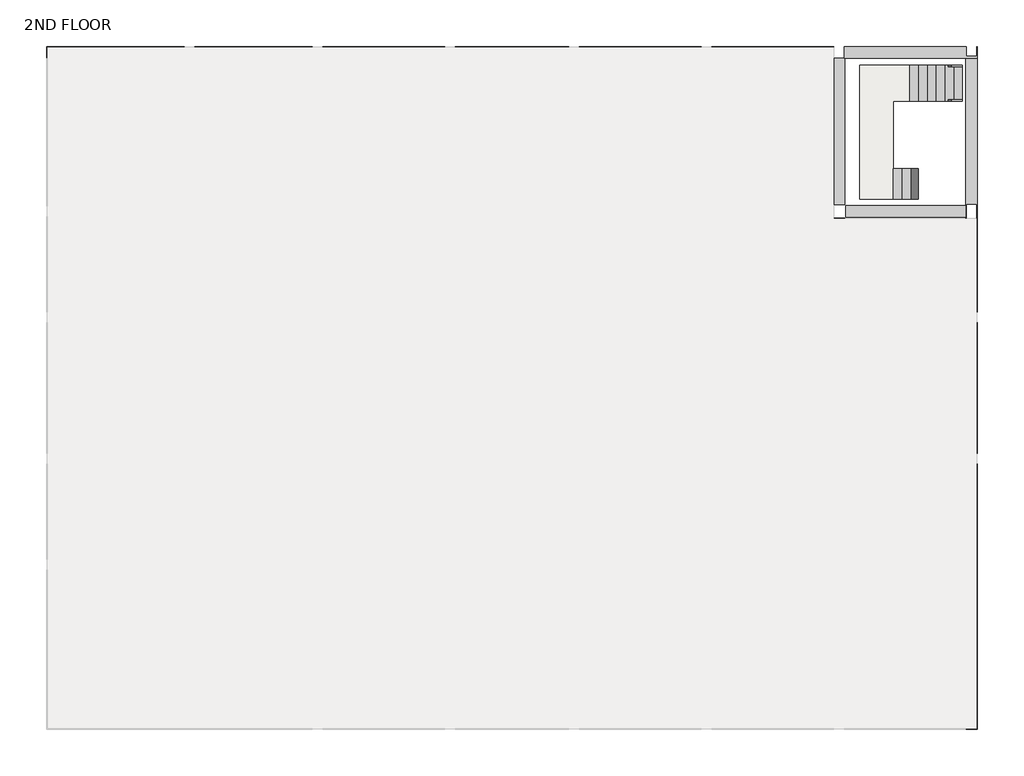
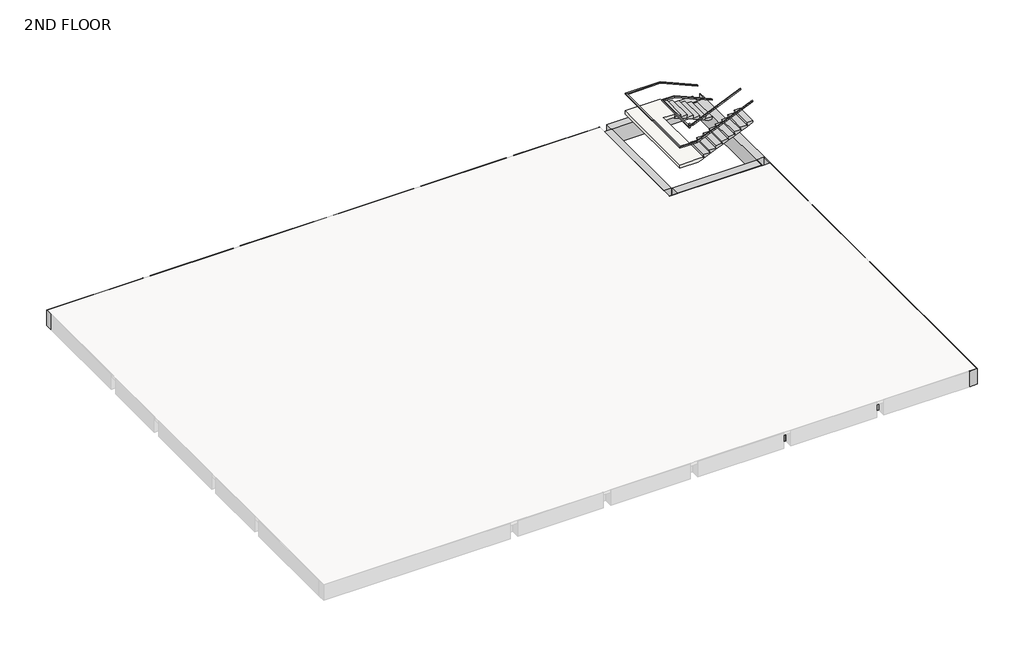
# One storey, part 2 of 2: 5 beams, 2 railings, 2 stair flights, 1 slab.
"""IFC4 building model written with IfcOpenShell, lengths in millimetres."""

from ifc_helpers import new_model, si_unit, frame, origin, place, context, project, spatial, polyline, outline, extrude, faceted_brep, element, save

model = new_model("IFC4")

# Units and contexts
model_context = context("Model", 3, world=origin())
ifc_project = project(units=[si_unit("LENGTHUNIT", "METRE", prefix="MILLI")], contexts=[model_context])

# Site, building, storey
site = spatial("IfcSite", under=ifc_project)
building = spatial("IfcBuilding", under=site)
storey = spatial("IfcBuildingStorey", under=building, Name="2ND FLOOR", Elevation=7620.0)

# Beams
placement = place(None, origin())
element("IfcBeam", 1, ObjectType="M_Concrete-Rectangular Beam : 400 x 800mm", at=placement, inside=storey, context=model_context, shape_type="Brep", body=[
    faceted_brep([(6397.6508981, 16716.9690835, 7620.0), (6397.6508981, 17116.9690835, 7620.0), (6375.4508981, 17116.9690835, 7620.0), (6375.4508981, 16789.9690835, 7620.0), (6019.8508981, 16789.9690835, 7620.0), (6019.8508981, 17116.9690835, 7620.0), (1803.4508981, 17116.9690835, 7620.0), (1803.4508981, 16716.9690835, 7620.0), (1825.6508981, 16716.9690835, 7620.0), (5997.6508981, 16716.9690835, 7620.0), (6397.6508981, 16716.9690835, 6820.0), (1803.4508981, 16716.9690835, 6820.0), (1825.6508981, 16716.9690835, 6820.0), (5997.6508981, 16716.9690835, 6820.0), (6397.6508981, 17116.9690835, 6820.0), (1803.4508981, 17116.9690835, 6820.0), (6019.8508981, 17116.9690835, 6820.0), (6019.8508981, 16789.9690835, 6820.0), (6375.4508981, 16789.9690835, 6820.0), (6375.4508981, 17116.9690835, 6820.0)], [[[0, 1, 2, 3, 4, 5, 6, 7, 8, 9]], [[10, 0, 9, 8, 7, 11, 12, 13]], [[14, 10, 13, 12, 11, 15, 16, 17, 18, 19]], [[1, 14, 19, 2]], [[1, 0, 10, 14]], [[18, 3, 2, 19]], [[3, 18, 17, 4]], [[4, 17, 16, 5]], [[5, 16, 15, 6]], [[7, 6, 15, 11]]]),
    faceted_brep([(-25701.5491019, 16716.9690835, 7620.0), (-25701.5491019, 17116.9690835, 7620.0), (-25701.5491019, 17116.9690835, 6820.0), (-25701.5491019, 16716.9690835, 6820.0), (-25323.7491019, 17094.7690835, 6820.0), (-25323.7491019, 16739.1690835, 6820.0), (-25323.7491019, 16739.1690835, 7467.6), (-25323.7491019, 17094.7690835, 7467.6), (-25679.3491019, 16739.1690835, 6820.0), (-25679.3491019, 16739.1690835, 7467.6), (-25679.3491019, 16716.9690835, 7620.0), (-25679.3491019, 16716.9690835, 7467.6), (-25679.3491019, 17094.7690835, 6820.0), (-25679.3491019, 17094.7690835, 7467.6), (-25679.3491019, 17094.7690835, 7620.0), (-20954.9491019, 16716.9690835, 6820.0), (-20954.9491019, 17116.9690835, 6820.0), (-20954.9491019, 17116.9690835, 7620.0), (-20954.9491019, 17094.7690835, 7620.0), (-20954.9491019, 17094.7690835, 7467.6), (-20954.9491019, 16716.9690835, 7467.6), (-25301.5491019, 16716.9690835, 6820.0), (-20977.1491019, 16716.9690835, 6820.0), (-20977.1491019, 16716.9690835, 7467.6), (-25301.5491019, 16716.9690835, 7467.6)], [[[0, 1, 2, 3]], [[4, 5, 6, 7]], [[5, 8, 9, 6]], [[10, 11, 9, 8, 12, 13, 14]], [[15, 16, 17, 18, 19, 20]], [[1, 0, 10, 14, 18, 17]], [[0, 3, 21, 22, 15, 20, 23, 24, 11, 10]], [[3, 2, 16, 15, 22, 21], [5, 4, 12, 8]], [[2, 1, 17, 16]], [[14, 13, 12, 4, 7, 19, 18]], [[19, 7, 6, 9, 11, 24, 23, 20]]]),
    faceted_brep([(-2768.5491019, 17094.7690835, 7467.6), (1447.8508981, 17094.7690835, 7467.6), (1447.8508981, 17094.7690835, 7620.0), (-2768.5491019, 17094.7690835, 7620.0), (-2768.5491019, 17116.9690835, 6820.0), (-2768.5491019, 16716.9690835, 6820.0), (-2768.5491019, 16716.9690835, 7467.6), (-2768.5491019, 17116.9690835, 7620.0), (1447.8508981, 16716.9690835, 6820.0), (1447.8508981, 17116.9690835, 6820.0), (1447.8508981, 17116.9690835, 7620.0), (1447.8508981, 16716.9690835, 7467.6), (-2746.3491019, 16716.9690835, 6820.0), (1425.6508981, 16716.9690835, 6820.0), (1425.6508981, 16716.9690835, 7467.6), (-2746.3491019, 16716.9690835, 7467.6)], [[[0, 1, 2, 3]], [[4, 5, 6, 0, 3, 7]], [[8, 9, 10, 2, 1, 11]], [[10, 7, 3, 2]], [[5, 12, 13, 8, 11, 14, 15, 6]], [[5, 4, 9, 8, 13, 12]], [[4, 7, 10, 9]], [[1, 0, 6, 15, 14, 11]]]),
    faceted_brep([(-16179.7491019, 17116.9690835, 6820.0), (-16179.7491019, 16716.9690835, 6820.0), (-16179.7491019, 16716.9690835, 7467.6), (-16179.7491019, 17094.7690835, 7467.6), (-16179.7491019, 17094.7690835, 7620.0), (-16179.7491019, 17116.9690835, 7620.0), (-11963.3491019, 16716.9690835, 6820.0), (-11963.3491019, 17116.9690835, 6820.0), (-11963.3491019, 17116.9690835, 7620.0), (-11963.3491019, 17094.7690835, 7620.0), (-11963.3491019, 17094.7690835, 7467.6), (-11963.3491019, 16716.9690835, 7467.6), (-16157.5491019, 16716.9690835, 6820.0), (-11985.5491019, 16716.9690835, 6820.0), (-11985.5491019, 16716.9690835, 7467.6), (-16157.5491019, 16716.9690835, 7467.6)], [[[0, 1, 2, 3, 4, 5]], [[6, 7, 8, 9, 10, 11]], [[8, 5, 4, 9]], [[1, 12, 13, 6, 11, 14, 15, 2]], [[1, 0, 7, 6, 13, 12]], [[0, 5, 8, 7]], [[3, 10, 9, 4]], [[10, 3, 2, 15, 14, 11]]]),
    faceted_brep([(-16535.3491019, 16716.9690835, 6820.0), (-16535.3491019, 17116.9690835, 6820.0), (-16535.3491019, 17116.9690835, 7620.0), (-16535.3491019, 17094.7690835, 7620.0), (-16535.3491019, 17094.7690835, 7467.6), (-16535.3491019, 16716.9690835, 7467.6), (-20599.3491019, 17116.9690835, 7620.0), (-20599.3491019, 17094.7690835, 7620.0), (-20599.3491019, 16716.9690835, 6820.0), (-20577.1491019, 16716.9690835, 6820.0), (-16557.5491019, 16716.9690835, 6820.0), (-16557.5491019, 16716.9690835, 7467.6), (-20577.1491019, 16716.9690835, 7467.6), (-20599.3491019, 16716.9690835, 7467.6), (-20599.3491019, 17116.9690835, 6820.0), (-20599.3491019, 17094.7690835, 7467.6)], [[[0, 1, 2, 3, 4, 5]], [[2, 6, 7, 3]], [[8, 9, 10, 0, 5, 11, 12, 13]], [[1, 0, 10, 9, 8, 14]], [[2, 1, 14, 6]], [[14, 8, 13, 15, 7, 6]], [[15, 4, 3, 7]], [[4, 15, 13, 12, 11, 5]]]),
    faceted_brep([(-11607.7491019, 17116.9690835, 6820.0), (-11607.7491019, 16716.9690835, 6820.0), (-11607.7491019, 16716.9690835, 7467.6), (-11607.7491019, 17094.7690835, 7467.6), (-11607.7491019, 17094.7690835, 7620.0), (-11607.7491019, 17116.9690835, 7620.0), (-7696.1491019, 16716.9690835, 6820.0), (-7696.1491019, 17116.9690835, 6820.0), (-7696.1491019, 17116.9690835, 7620.0), (-7696.1491019, 17094.7690835, 7620.0), (-7696.1491019, 17094.7690835, 7467.6), (-7696.1491019, 16716.9690835, 7467.6), (-11585.5491019, 16716.9690835, 6820.0), (-7718.3491019, 16716.9690835, 6820.0), (-7718.3491019, 16716.9690835, 7467.6), (-11585.5491019, 16716.9690835, 7467.6)], [[[0, 1, 2, 3, 4, 5]], [[6, 7, 8, 9, 10, 11]], [[8, 5, 4, 9]], [[1, 12, 13, 6, 11, 14, 15, 2]], [[1, 0, 7, 6, 13, 12]], [[0, 5, 8, 7]], [[3, 10, 9, 4]], [[10, 3, 2, 15, 14, 11]]]),
    faceted_brep([(-7340.5491019, 17116.9690835, 6820.0), (-7340.5491019, 16716.9690835, 6820.0), (-7340.5491019, 16716.9690835, 7467.6), (-7340.5491019, 17094.7690835, 7467.6), (-7340.5491019, 17094.7690835, 7620.0), (-7340.5491019, 17116.9690835, 7620.0), (-3124.1491019, 16716.9690835, 6820.0), (-3124.1491019, 17116.9690835, 6820.0), (-3124.1491019, 17116.9690835, 7620.0), (-3124.1491019, 17094.7690835, 7620.0), (-3124.1491019, 17094.7690835, 7467.6), (-3124.1491019, 16716.9690835, 7467.6), (-7318.3491019, 16716.9690835, 6820.0), (-3146.3491019, 16716.9690835, 6820.0), (-3146.3491019, 16716.9690835, 7467.6), (-7318.3491019, 16716.9690835, 7467.6)], [[[0, 1, 2, 3, 4, 5]], [[6, 7, 8, 9, 10, 11]], [[8, 5, 4, 9]], [[1, 12, 13, 6, 11, 14, 15, 2]], [[1, 0, 7, 6, 13, 12]], [[0, 5, 8, 7]], [[3, 10, 9, 4]], [[10, 3, 2, 15, 14, 11]]]),
])
element("IfcBeam", 2, ObjectType="M_Concrete-Rectangular Beam : 400 x 800mm", at=placement, inside=storey, context=model_context, shape_type="Brep", body=[
    faceted_brep([(5997.6508981, -6447.8309165, 7620.0), (6397.6508981, -6447.8309165, 7620.0), (6397.6508981, 2718.3690835, 7620.0), (6375.4508981, 2718.3690835, 7620.0), (6375.4508981, -6425.6309165, 7620.0), (5997.6508981, -6425.6309165, 7620.0), (5997.6508981, -6447.8309165, 6820.0), (5997.6508981, -6425.6309165, 7467.6), (5997.6508981, -6047.8309165, 7467.6), (5997.6508981, -961.4309165, 7467.6), (5997.6508981, -561.4309165, 7467.6), (5997.6508981, 2696.1690835, 7467.6), (5997.6508981, 2718.3690835, 7467.6), (5997.6508981, 2718.3690835, 6820.0), (5997.6508981, 2696.1690835, 6820.0), (5997.6508981, -561.4309165, 6820.0), (5997.6508981, -961.4309165, 6820.0), (5997.6508981, -6047.8309165, 6820.0), (6397.6508981, -6447.8309165, 6820.0), (6397.6508981, 2718.3690835, 6820.0), (6375.4508981, -6425.6309165, 6820.0), (6375.4508981, -6070.0309165, 6820.0), (6019.8508981, -6070.0309165, 6820.0), (6019.8508981, -6425.6309165, 6820.0), (6375.4508981, -1015.4309165, 6820.0), (6375.4508981, -507.4309165, 6820.0), (6019.8508981, -507.4309165, 6820.0), (6019.8508981, -1015.4309165, 6820.0), (6375.4508981, 2718.3690835, 7467.6), (6375.4508981, -507.4309165, 7467.6), (6375.4508981, -1015.4309165, 7467.6), (6375.4508981, -6070.0309165, 7467.6), (6375.4508981, -6425.6309165, 7467.6), (6019.8508981, -6425.6309165, 7467.6), (6019.8508981, -6070.0309165, 7467.6), (6019.8508981, -1015.4309165, 7467.6), (6019.8508981, -507.4309165, 7467.6)], [[[0, 1, 2, 3, 4, 5]], [[6, 0, 5, 7, 8, 9, 10, 11, 12, 13, 14, 15, 16, 17]], [[18, 6, 17, 16, 15, 14, 13, 19], [20, 21, 22, 23], [24, 25, 26, 27]], [[1, 18, 19, 2]], [[1, 0, 6, 18]], [[3, 28, 29, 25, 24, 30, 31, 21, 20, 32, 4]], [[4, 32, 20, 23, 33, 7, 5]], [[23, 22, 34, 33]], [[22, 21, 31, 34]], [[19, 13, 12, 28, 3, 2]], [[24, 27, 35, 30]], [[27, 26, 36, 35]], [[26, 25, 29, 36]], [[31, 30, 35, 36, 29, 28, 12, 11, 10, 9, 8, 7, 33, 34]]]),
    faceted_brep([(5997.6508981, 16716.9690835, 6820.0), (5997.6508981, 16716.9690835, 7620.0), (6397.6508981, 16716.9690835, 7620.0), (6397.6508981, 16716.9690835, 6820.0), (5997.6508981, 7950.7690835, 6820.0), (6397.6508981, 7950.7690835, 6820.0), (6397.6508981, 7950.7690835, 7620.0), (6375.4508981, 7950.7690835, 7620.0), (6375.4508981, 7950.7690835, 7467.6), (5997.6508981, 7950.7690835, 7467.6), (5997.6508981, 11630.5690835, 7620.0), (5997.6508981, 11230.5690835, 7620.0), (5997.6508981, 11176.5690835, 7620.0), (6019.8508981, 11176.5690835, 7620.0), (6019.8508981, 11684.5690835, 7620.0), (6375.4508981, 11684.5690835, 7620.0), (6375.4508981, 11176.5690835, 7620.0), (5997.6508981, 11630.5690835, 6820.0), (5997.6508981, 11230.5690835, 6820.0), (5997.6508981, 7972.9690835, 6820.0), (5997.6508981, 7972.9690835, 7467.6), (5997.6508981, 11176.5690835, 7467.6), (6375.4508981, 11176.5690835, 6820.0), (6375.4508981, 11684.5690835, 6820.0), (6019.8508981, 11684.5690835, 6820.0), (6019.8508981, 11176.5690835, 6820.0), (6019.8508981, 11176.5690835, 7467.6), (6375.4508981, 11176.5690835, 7467.6)], [[[0, 1, 2, 3]], [[4, 5, 6, 7, 8, 9]], [[2, 1, 10, 11, 12, 13, 14, 15, 16, 7, 6]], [[1, 0, 17, 18, 19, 4, 9, 20, 21, 12, 11, 10]], [[0, 3, 5, 4, 19, 18, 17], [22, 23, 24, 25]], [[3, 2, 6, 5]], [[22, 25, 26, 27]], [[24, 14, 13, 26, 25]], [[14, 24, 23, 15]], [[8, 27, 26, 21, 20, 9]], [[27, 8, 7, 16, 15, 23, 22]], [[21, 26, 13, 12]]]),
    faceted_brep([(6397.6508981, 7595.1690835, 6820.0), (5997.6508981, 7595.1690835, 6820.0), (5997.6508981, 7595.1690835, 7467.6), (6375.4508981, 7595.1690835, 7467.6), (6375.4508981, 7595.1690835, 7620.0), (6397.6508981, 7595.1690835, 7620.0), (5997.6508981, 3073.9690835, 6820.0), (6397.6508981, 3073.9690835, 6820.0), (6397.6508981, 3073.9690835, 7620.0), (6375.4508981, 3073.9690835, 7620.0), (6375.4508981, 3073.9690835, 7467.6), (5997.6508981, 3073.9690835, 7467.6), (5997.6508981, 7572.9690835, 6820.0), (5997.6508981, 3096.1690835, 6820.0), (5997.6508981, 3096.1690835, 7467.6), (5997.6508981, 7572.9690835, 7467.6)], [[[0, 1, 2, 3, 4, 5]], [[6, 7, 8, 9, 10, 11]], [[8, 5, 4, 9]], [[1, 12, 13, 6, 11, 14, 15, 2]], [[1, 0, 7, 6, 13, 12]], [[0, 5, 8, 7]], [[3, 10, 9, 4]], [[10, 3, 2, 15, 14, 11]]]),
])
element("IfcBeam", 3, ObjectType="M_Concrete-Rectangular Beam : 400 x 800mm", at=placement, inside=storey, context=model_context, shape_type="SweptSolid", body=[
    extrude(outline(polyline([(-2746.3491019, -6047.8309165), (-2768.5491019, -6047.8309165), (-2768.5491019, -6019.2309165), (-3124.1491019, -6019.2309165), (-3124.1491019, -6047.8309165), (-3146.3491019, -6047.8309165), (-3146.3491019, -990.0309165), (-2746.3491019, -990.0309165), (-2746.3491019, -6047.8309165)])), frame((0.0, 0.0, 6820.0), z_axis=(0.0, 0.0, 1.0), x_axis=(1.0, 0.0, 0.0)), (0.0, 0.0, 1.0), 647.6),
    extrude(outline(polyline([(-2768.5491019, 16716.9690835), (-2746.3491019, 16716.9690835), (-2746.3491019, 11659.1690835), (-3146.3491019, 11659.1690835), (-3146.3491019, 16716.9690835), (-3124.1491019, 16716.9690835), (-3124.1491019, 16688.3690835), (-2768.5491019, 16688.3690835), (-2768.5491019, 16716.9690835)])), frame((0.0, 0.0, 6820.0), z_axis=(0.0, 0.0, 1.0), x_axis=(1.0, 0.0, 0.0)), (0.0, 0.0, 1.0), 647.6),
    extrude(outline(polyline([(-3146.3491019, 11201.9690835), (-2746.3491019, 11201.9690835), (-2746.3491019, 8001.5690835), (-3146.3491019, 8001.5690835), (-3146.3491019, 11201.9690835)])), frame((0.0, 0.0, 6820.0), z_axis=(0.0, 0.0, 1.0), x_axis=(1.0, 0.0, 0.0)), (0.0, 0.0, 1.0), 647.6),
    extrude(outline(polyline([(-3146.3491019, 7544.3690835), (-2746.3491019, 7544.3690835), (-2746.3491019, 3124.7690835), (-3146.3491019, 3124.7690835), (-3146.3491019, 7544.3690835)])), frame((0.0, 0.0, 6820.0), z_axis=(0.0, 0.0, 1.0), x_axis=(1.0, 0.0, 0.0)), (0.0, 0.0, 1.0), 647.6),
    extrude(outline(polyline([(-2746.3491019, -532.8309165), (-3146.3491019, -532.8309165), (-3146.3491019, 2667.5690835), (-2746.3491019, 2667.5690835), (-2746.3491019, -532.8309165)])), frame((0.0, 0.0, 6820.0), z_axis=(0.0, 0.0, 1.0), x_axis=(1.0, 0.0, 0.0)), (0.0, 0.0, 1.0), 647.6),
])
element("IfcBeam", 4, ObjectType="M_Concrete-Rectangular Beam : 400 x 800mm", at=placement, inside=storey, context=model_context, shape_type="Brep", body=[
    faceted_brep([(1425.6508981, -990.0309165, 6820.0), (1425.6508981, -6047.8309165, 6820.0), (1425.6508981, -6047.8309165, 7467.6), (1425.6508981, -990.0309165, 7467.6), (1825.6508981, -6047.8309165, 6820.0), (1803.4508981, -6047.8309165, 6820.0), (1803.4508981, -6019.2309165, 6820.0), (1447.8508981, -6019.2309165, 6820.0), (1447.8508981, -6047.8309165, 6820.0), (1825.6508981, -990.0309165, 6820.0), (1825.6508981, -990.0309165, 7467.6), (1825.6508981, -6047.8309165, 7467.6), (1447.8508981, -6047.8309165, 7467.6), (1803.4508981, -6047.8309165, 7467.6), (1803.4508981, -6019.2309165, 7467.6), (1447.8508981, -6019.2309165, 7467.6)], [[[0, 1, 2, 3]], [[4, 5, 6, 7, 8, 1, 0, 9]], [[4, 9, 10, 11]], [[1, 8, 12, 2]], [[6, 5, 13, 14]], [[8, 7, 15, 12]], [[7, 6, 14, 15]], [[5, 4, 11, 13]], [[9, 0, 3, 10]], [[3, 2, 12, 15, 14, 13, 11, 10]]]),
    faceted_brep([(1825.6508981, 16716.9690835, 7620.0), (1825.6508981, 16716.9690835, 6820.0), (1803.4508981, 16716.9690835, 6820.0), (1803.4508981, 16716.9690835, 7620.0), (1803.4508981, 16713.7690835, 6820.0), (1803.4508981, 16713.7690835, 7620.0), (1447.8508981, 16713.7690835, 6820.0), (1447.8508981, 16713.7690835, 7467.6), (1447.8508981, 16713.7690835, 7620.0), (1447.8508981, 16716.9690835, 6820.0), (1447.8508981, 16716.9690835, 7467.6), (1425.6508981, 16716.9690835, 6820.0), (1425.6508981, 16716.9690835, 7467.6), (1425.6508981, 11659.1690835, 6820.0), (1825.6508981, 11659.1690835, 6820.0), (1825.6508981, 11659.1690835, 7620.0), (1447.8508981, 11659.1690835, 7620.0), (1447.8508981, 11659.1690835, 7467.6), (1425.6508981, 11659.1690835, 7467.6)], [[[0, 1, 2, 3]], [[4, 5, 3, 2]], [[5, 4, 6, 7, 8]], [[6, 9, 10, 7]], [[9, 11, 12, 10]], [[13, 14, 15, 16, 17, 18]], [[0, 3, 5, 8, 16, 15]], [[11, 13, 18, 12]], [[2, 1, 14, 13, 11, 9, 6, 4]], [[1, 0, 15, 14]], [[17, 7, 10, 12, 18]], [[7, 17, 16, 8]]]),
    faceted_brep([(1825.6508981, 11201.9690835, 6820.0), (1425.6508981, 11201.9690835, 6820.0), (1425.6508981, 11201.9690835, 7467.6), (1447.8508981, 11201.9690835, 7467.6), (1447.8508981, 11201.9690835, 7620.0), (1825.6508981, 11201.9690835, 7620.0), (1425.6508981, 8001.5690835, 6820.0), (1825.6508981, 8001.5690835, 6820.0), (1825.6508981, 8001.5690835, 7467.6), (1425.6508981, 8001.5690835, 7467.6), (1447.8508981, 11176.5690835, 7620.0), (1825.6508981, 11176.5690835, 7620.0), (1825.6508981, 11176.5690835, 7467.6), (1447.8508981, 11176.5690835, 7467.6)], [[[0, 1, 2, 3, 4, 5]], [[6, 7, 8, 9]], [[5, 4, 10, 11]], [[1, 6, 9, 2]], [[1, 0, 7, 6]], [[0, 5, 11, 12, 8, 7]], [[12, 13, 3, 2, 9, 8]], [[13, 10, 4, 3]], [[10, 13, 12, 11]]]),
    faceted_brep([(1825.6508981, 7544.3690835, 6820.0), (1425.6508981, 7544.3690835, 6820.0), (1425.6508981, 7544.3690835, 7467.6), (1825.6508981, 7544.3690835, 7467.6), (1425.6508981, 3124.7690835, 6820.0), (1825.6508981, 3124.7690835, 6820.0), (1825.6508981, 3124.7690835, 7467.6), (1425.6508981, 3124.7690835, 7467.6)], [[[0, 1, 2, 3]], [[4, 5, 6, 7]], [[1, 4, 7, 2]], [[1, 0, 5, 4]], [[5, 0, 3, 6]], [[3, 2, 7, 6]]]),
    faceted_brep([(1425.6508981, -532.8309165, 6820.0), (1825.6508981, -532.8309165, 6820.0), (1825.6508981, -532.8309165, 7467.6), (1425.6508981, -532.8309165, 7467.6), (1425.6508981, 2667.5690835, 6820.0), (1425.6508981, 2667.5690835, 7467.6), (1825.6508981, 2667.5690835, 6820.0), (1825.6508981, 2667.5690835, 7467.6)], [[[0, 1, 2, 3]], [[4, 0, 3, 5]], [[1, 0, 4, 6]], [[1, 6, 7, 2]], [[6, 4, 5, 7]], [[3, 2, 7, 5]]]),
])
element("IfcBeam", 5, ObjectType="M_Concrete-Rectangular Beam : 400 x 800mm", at=placement, inside=storey, context=model_context, shape_type="SweptSolid", body=[
    extrude(outline(polyline([(-25301.5491019, 11608.3690835), (-25301.5491019, 11630.5690835), (-21005.7491019, 11630.5690835), (-21005.7491019, 11230.5690835), (-25301.5491019, 11230.5690835), (-25301.5491019, 11252.7690835), (-25247.5491019, 11252.7690835), (-25247.5491019, 11608.3690835), (-25301.5491019, 11608.3690835)])), frame((0.0, 0.0, 6820.0), z_axis=(0.0, 0.0, 1.0), x_axis=(1.0, 0.0, 0.0)), (0.0, 0.0, 1.0), 647.6),
    extrude(outline(polyline([(5997.6508981, 11630.5690835), (5997.6508981, 11230.5690835), (1854.2508981, 11230.5690835), (1854.2508981, 11630.5690835), (5997.6508981, 11630.5690835)])), frame((0.0, 0.0, 6820.0), z_axis=(0.0, 0.0, 1.0), x_axis=(1.0, 0.0, 0.0)), (0.0, 0.0, 1.0), 800.0),
    extrude(outline(polyline([(-20548.5491019, 11230.5690835), (-20548.5491019, 11630.5690835), (-16586.1491019, 11630.5690835), (-16586.1491019, 11230.5690835), (-20548.5491019, 11230.5690835)])), frame((0.0, 0.0, 6820.0), z_axis=(0.0, 0.0, 1.0), x_axis=(1.0, 0.0, 0.0)), (0.0, 0.0, 1.0), 647.6),
    extrude(outline(polyline([(-16128.9491019, 11230.5690835), (-16128.9491019, 11630.5690835), (-12014.1491019, 11630.5690835), (-12014.1491019, 11230.5690835), (-16128.9491019, 11230.5690835)])), frame((0.0, 0.0, 6820.0), z_axis=(0.0, 0.0, 1.0), x_axis=(1.0, 0.0, 0.0)), (0.0, 0.0, 1.0), 647.6),
    extrude(outline(polyline([(-11556.9491019, 11230.5690835), (-11556.9491019, 11630.5690835), (-7746.9491019, 11630.5690835), (-7746.9491019, 11230.5690835), (-11556.9491019, 11230.5690835)])), frame((0.0, 0.0, 6820.0), z_axis=(0.0, 0.0, 1.0), x_axis=(1.0, 0.0, 0.0)), (0.0, 0.0, 1.0), 647.6),
    extrude(outline(polyline([(-7289.7491019, 11230.5690835), (-7289.7491019, 11630.5690835), (-3174.9491019, 11630.5690835), (-3174.9491019, 11230.5690835), (-7289.7491019, 11230.5690835)])), frame((0.0, 0.0, 6820.0), z_axis=(0.0, 0.0, 1.0), x_axis=(1.0, 0.0, 0.0)), (0.0, 0.0, 1.0), 647.6),
    extrude(outline(polyline([(-2717.7491019, 11230.5690835), (-2717.7491019, 11630.5690835), (1397.0508981, 11630.5690835), (1397.0508981, 11230.5690835), (-2717.7491019, 11230.5690835)])), frame((0.0, 0.0, 6820.0), z_axis=(0.0, 0.0, 1.0), x_axis=(1.0, 0.0, 0.0)), (0.0, 0.0, 1.0), 647.6),
])

# Railings
element("IfcRailing", 6, ObjectType="Handrail", at=placement, inside=storey, context=model_context, shape_type="Brep", body=[
    faceted_brep([(5878.2258195, 16426.305974, 8664.575), (5878.2258195, 16426.305974, 8609.3359813), (5878.2258195, 16477.105974, 8609.3359813), (5878.2258195, 16477.105974, 8664.575), (4049.4258195, 16426.305974, 9445.625), (4039.0320197, 16426.305974, 9394.825), (4039.0320197, 16477.105974, 9394.825), (4049.4258195, 16477.105974, 9445.625), (2398.4258195, 16426.305974, 9445.625), (2398.4258195, 16426.305974, 9394.825), (2347.6258195, 16477.105974, 9394.825), (2347.6258195, 16477.105974, 9445.625), (2398.4258195, 11896.1816424, 9445.625), (2398.4258195, 11896.1816424, 9394.825), (2347.6258195, 11845.3816424, 9394.825), (2347.6258195, 11845.3816424, 9445.625), (3188.2923097, 11896.1816424, 9445.625), (3198.6861096, 11896.1816424, 9394.825), (3198.6861096, 11845.3816424, 9394.825), (3188.2923097, 11845.3816424, 9445.625), (5931.4923097, 11896.1816424, 10617.2), (5931.4923097, 11845.3816424, 10617.2), (5931.4923097, 11845.3816424, 10561.9609813), (5931.4923097, 11896.1816424, 10561.9609813)], [[[0, 1, 2, 3]], [[1, 0, 4, 5]], [[2, 1, 5, 6]], [[3, 2, 6, 7]], [[0, 3, 7, 4]], [[5, 4, 8, 9]], [[6, 5, 9, 10]], [[7, 6, 10, 11]], [[4, 7, 11, 8]], [[9, 8, 12, 13]], [[10, 9, 13, 14]], [[11, 10, 14, 15]], [[8, 11, 15, 12]], [[13, 12, 16, 17]], [[14, 13, 17, 18]], [[15, 14, 18, 19]], [[12, 15, 19, 16]], [[20, 21, 22, 23]], [[17, 16, 20, 23]], [[18, 17, 23, 22]], [[19, 18, 22, 21]], [[16, 19, 21, 20]]]),
])
element("IfcRailing", 7, ObjectType="Handrail", at=placement, inside=storey, context=model_context, shape_type="Brep", body=[
    faceted_brep([(5878.2258195, 15223.6852874, 8664.575), (5878.2258195, 15223.6852874, 8609.3359813), (5878.2258195, 15274.4852874, 8609.3359813), (5878.2258195, 15274.4852874, 8664.575), (4049.4258195, 15223.6852874, 9445.625), (4039.0320197, 15223.6852874, 9394.825), (4039.0320197, 15274.4852874, 9394.825), (4049.4258195, 15274.4852874, 9445.625), (3493.0923097, 15223.6852874, 9445.625), (3493.0923097, 15223.6852874, 9394.825), (3442.2923097, 15274.4852874, 9394.825), (3442.2923097, 15274.4852874, 9445.625), (3493.0923097, 12985.9409784, 9445.625), (3493.0923097, 12935.1409784, 9394.825), (3442.2923097, 12935.1409784, 9394.825), (3442.2923097, 12985.9409784, 9445.625), (3493.0923097, 12985.9409784, 9608.34375), (3493.0923097, 12935.1409784, 9557.54375), (3442.2923097, 12935.1409784, 9557.54375), (3442.2923097, 12985.9409784, 9608.34375), (3493.0923097, 12909.7409784, 9608.34375), (3493.0923097, 12909.7409784, 9557.54375), (3442.2923097, 12858.9409784, 9557.54375), (3442.2923097, 12858.9409784, 9608.34375), (3569.2923097, 12909.7409784, 9608.34375), (3579.6861096, 12909.7409784, 9557.54375), (3579.6861096, 12858.9409784, 9557.54375), (3569.2923097, 12858.9409784, 9608.34375), (5931.4923097, 12909.7409784, 10617.2), (5931.4923097, 12858.9409784, 10617.2), (5931.4923097, 12858.9409784, 10561.9609813), (5931.4923097, 12909.7409784, 10561.9609813)], [[[0, 1, 2, 3]], [[1, 0, 4, 5]], [[2, 1, 5, 6]], [[3, 2, 6, 7]], [[0, 3, 7, 4]], [[5, 4, 8, 9]], [[6, 5, 9, 10]], [[7, 6, 10, 11]], [[4, 7, 11, 8]], [[9, 8, 12, 13]], [[10, 9, 13, 14]], [[11, 10, 14, 15]], [[8, 11, 15, 12]], [[13, 12, 16, 17]], [[14, 13, 17, 18]], [[15, 14, 18, 19]], [[12, 15, 19, 16]], [[17, 16, 20, 21]], [[18, 17, 21, 22]], [[19, 18, 22, 23]], [[16, 19, 23, 20]], [[21, 20, 24, 25]], [[22, 21, 25, 26]], [[23, 22, 26, 27]], [[20, 23, 27, 24]], [[28, 29, 30, 31]], [[25, 24, 28, 31]], [[26, 25, 31, 30]], [[27, 26, 30, 29]], [[24, 27, 29, 28]]]),
])

# Slab
element("IfcSlab", 8, ObjectType="7\" Thickness", at=placement, inside=storey, context=model_context, shape_type="Brep", body=[
    faceted_brep([(4049.4258195, 16477.105974, 8531.225), (4049.4258195, 15223.6852874, 8531.225), (4030.3758195, 15223.6852874, 8401.05), (4030.3758195, 16477.105974, 8401.05), (2347.6258195, 16477.105974, 8531.225), (2347.6258195, 11845.3816424, 8531.225), (3257.5052912, 11845.3816424, 8531.225), (3493.0923097, 11845.3816424, 8531.225), (3512.1423097, 11845.3816424, 8531.225), (3512.1423097, 12909.7409784, 8531.225), (3493.0923097, 12909.7409784, 8531.225), (3493.0923097, 15223.6852874, 8531.225), (3980.212838, 15223.6852874, 8531.225), (3980.212838, 16477.105974, 8531.225), (4030.3758195, 15223.6852874, 8332.0012267), (4030.3758195, 16477.105974, 8332.0012267), (3980.212838, 16477.105974, 8353.425), (2347.6258195, 16477.105974, 8353.425), (2347.6258195, 11845.3816424, 8353.425), (3257.5052912, 11845.3816424, 8353.425), (3493.0923097, 11845.3816424, 8454.0402892), (3512.1423097, 11845.3816424, 8462.1762267), (3512.1423097, 12909.7409784, 8462.1762267), (3493.0923097, 12909.7409784, 8454.0402892), (3493.0923097, 12909.7409784, 8353.425), (3493.0923097, 15223.6852874, 8353.425), (3980.212838, 15223.6852874, 8353.425), (3257.5052912, 12909.7409784, 8353.425)], [[[0, 1, 2, 3]], [[4, 5, 6, 7, 8, 9, 10, 11, 12, 1, 0, 13]], [[3, 2, 14, 15]], [[0, 3, 15, 16, 17, 4, 13]], [[5, 4, 17, 18]], [[5, 18, 19, 20, 7, 6]], [[8, 7, 20, 21]], [[9, 8, 21, 22]], [[10, 9, 22, 23]], [[11, 10, 23, 24, 25]], [[2, 1, 12, 11, 25, 26, 14]], [[24, 27, 19, 18, 17, 16, 26, 25]], [[27, 24, 23]], [[26, 16, 15, 14]], [[19, 27, 23, 22, 21, 20]]]),
])

# Stair flights
element("IfcStairFlight", 9, ObjectType="3/4\" Nosing", at=placement, inside=storey, context=model_context, shape_type="Brep", body=[
    faceted_brep([(5878.2258195, 16477.105974, 7750.175), (5878.2258195, 15223.6852874, 7750.175), (5859.1758195, 15223.6852874, 7620.0), (5859.1758195, 16477.105974, 7620.0), (5554.3758195, 16477.105974, 7750.175), (5554.3758195, 15223.6852874, 7750.175), (5554.3758195, 15223.6852874, 7681.1262267), (5697.5006429, 15223.6852874, 7620.0), (5697.5006429, 16477.105974, 7620.0), (5554.3758195, 16477.105974, 7681.1262267), (5573.4258195, 15223.6852874, 7880.35), (5573.4258195, 16477.105974, 7880.35), (5249.5758195, 16477.105974, 7880.35), (5249.5758195, 15223.6852874, 7880.35), (5249.5758195, 15223.6852874, 7811.3012267), (5249.5758195, 16477.105974, 7811.3012267), (5268.6258195, 15223.6852874, 8010.525), (5268.6258195, 16477.105974, 8010.525), (4944.7758195, 16477.105974, 8010.525), (4944.7758195, 15223.6852874, 8010.525), (4944.7758195, 15223.6852874, 7941.4762267), (4944.7758195, 16477.105974, 7941.4762267), (4963.8258195, 15223.6852874, 8140.7), (4963.8258195, 16477.105974, 8140.7), (4639.9758195, 16477.105974, 8140.7), (4639.9758195, 15223.6852874, 8140.7), (4639.9758195, 15223.6852874, 8071.6512267), (4639.9758195, 16477.105974, 8071.6512267), (4659.0258195, 15223.6852874, 8270.875), (4659.0258195, 16477.105974, 8270.875), (4335.1758195, 16477.105974, 8270.875), (4335.1758195, 15223.6852874, 8270.875), (4335.1758195, 15223.6852874, 8201.8262267), (4335.1758195, 16477.105974, 8201.8262267), (4030.3758195, 15223.6852874, 8401.05), (4049.4258195, 15223.6852874, 8401.05), (4354.2258195, 15223.6852874, 8401.05), (4354.2258195, 16477.105974, 8401.05), (4049.4258195, 16477.105974, 8401.05), (4030.3758195, 16477.105974, 8401.05), (4030.3758195, 15223.6852874, 8332.0012267), (4049.4258195, 15223.6852874, 8323.8652892), (4049.4258195, 16477.105974, 8323.8652892), (4030.3758195, 16477.105974, 8332.0012267)], [[[0, 1, 2, 3]], [[1, 0, 4, 5]], [[1, 5, 6, 7, 2]], [[4, 0, 3, 8, 9]], [[10, 11, 12, 13]], [[10, 13, 14, 6, 5]], [[12, 11, 4, 9, 15]], [[5, 4, 11, 10]], [[16, 17, 18, 19]], [[16, 19, 20, 14, 13]], [[18, 17, 12, 15, 21]], [[13, 12, 17, 16]], [[22, 23, 24, 25]], [[22, 25, 26, 20, 19]], [[24, 23, 18, 21, 27]], [[19, 18, 23, 22]], [[28, 29, 30, 31]], [[28, 31, 32, 26, 25]], [[30, 29, 24, 27, 33]], [[25, 24, 29, 28]], [[34, 35, 36, 37, 38, 39]], [[35, 34, 40, 41]], [[38, 37, 30, 33, 42]], [[34, 39, 43, 40]], [[31, 30, 37, 36]], [[3, 2, 7, 8]], [[8, 7, 6, 14, 20, 26, 32, 41, 40, 43, 42, 33, 27, 21, 15, 9]], [[36, 35, 41, 32, 31]], [[39, 38, 42, 43]]]),
])
element("IfcStairFlight", 10, ObjectType="3/4\" Nosing", at=placement, inside=storey, context=model_context, shape_type="Brep", body=[
    faceted_brep([(3493.0923097, 11845.3816424, 8661.4), (3493.0923097, 12909.7409784, 8661.4), (3512.1423097, 12909.7409784, 8531.225), (3512.1423097, 11845.3816424, 8531.225), (3816.9423097, 11845.3816424, 8661.4), (3816.9423097, 12909.7409784, 8661.4), (3816.9423097, 12909.7409784, 8592.3512267), (3512.1423097, 12909.7409784, 8462.1762267), (3512.1423097, 11845.3816424, 8462.1762267), (3816.9423097, 11845.3816424, 8592.3512267), (3797.8923097, 12909.7409784, 8791.575), (3797.8923097, 11845.3816424, 8791.575), (4121.7423097, 11845.3816424, 8791.575), (4121.7423097, 12909.7409784, 8791.575), (4121.7423097, 12909.7409784, 8722.5262267), (4121.7423097, 11845.3816424, 8722.5262267), (4102.6923097, 12909.7409784, 8921.75), (4102.6923097, 11845.3816424, 8921.75), (4426.5423097, 11845.3816424, 8921.75), (4426.5423097, 12909.7409784, 8921.75), (4426.5423097, 12909.7409784, 8852.7012267), (4426.5423097, 11845.3816424, 8852.7012267), (4407.4923097, 12909.7409784, 9051.925), (4407.4923097, 11845.3816424, 9051.925), (4731.3423097, 11845.3816424, 9051.925), (4731.3423097, 12909.7409784, 9051.925), (4731.3423097, 12909.7409784, 8982.8762267), (4731.3423097, 11845.3816424, 8982.8762267), (4712.2923097, 12909.7409784, 9182.1), (4712.2923097, 11845.3816424, 9182.1), (5036.1423097, 11845.3816424, 9182.1), (5036.1423097, 12909.7409784, 9182.1), (5036.1423097, 12909.7409784, 9113.0512267), (5036.1423097, 11845.3816424, 9113.0512267), (5017.0923097, 12909.7409784, 9312.275), (5017.0923097, 11845.3816424, 9312.275), (5340.9423097, 11845.3816424, 9312.275), (5340.9423097, 12909.7409784, 9312.275), (5340.9423097, 12909.7409784, 9243.2262267), (5340.9423097, 11845.3816424, 9243.2262267), (5321.8923097, 12909.7409784, 9442.45), (5321.8923097, 11845.3816424, 9442.45), (5645.7423097, 11845.3816424, 9442.45), (5645.7423097, 12909.7409784, 9442.45), (5645.7423097, 12909.7409784, 9373.4012267), (5645.7423097, 11845.3816424, 9373.4012267), (5626.6923097, 12909.7409784, 9572.625), (5626.6923097, 11845.3816424, 9572.625), (5931.4923097, 11845.3816424, 9572.625), (5931.4923097, 12909.7409784, 9572.625), (5931.4923097, 12909.7409784, 9495.4402892), (5931.4923097, 11845.3816424, 9495.4402892)], [[[0, 1, 2, 3]], [[1, 0, 4, 5]], [[1, 5, 6, 7, 2]], [[3, 2, 7, 8]], [[4, 0, 3, 8, 9]], [[10, 11, 12, 13]], [[10, 13, 14, 6, 5]], [[12, 11, 4, 9, 15]], [[11, 10, 5, 4]], [[16, 17, 18, 19]], [[16, 19, 20, 14, 13]], [[18, 17, 12, 15, 21]], [[17, 16, 13, 12]], [[22, 23, 24, 25]], [[22, 25, 26, 20, 19]], [[24, 23, 18, 21, 27]], [[23, 22, 19, 18]], [[28, 29, 30, 31]], [[28, 31, 32, 26, 25]], [[30, 29, 24, 27, 33]], [[29, 28, 25, 24]], [[34, 35, 36, 37]], [[34, 37, 38, 32, 31]], [[36, 35, 30, 33, 39]], [[35, 34, 31, 30]], [[40, 41, 42, 43]], [[40, 43, 44, 38, 37]], [[42, 41, 36, 39, 45]], [[41, 40, 37, 36]], [[46, 47, 48, 49]], [[46, 49, 50, 44, 43]], [[48, 47, 42, 45, 51]], [[49, 48, 51, 50]], [[47, 46, 43, 42]], [[7, 6, 14, 20, 26, 32, 38, 44, 50, 51, 45, 39, 33, 27, 21, 15, 9, 8]]]),
])

save(model, "model.ifc")

# Revit data of these elements
# Type "M_Concrete-Rectangular Beam : 400 x 800mm"
#   Length [instance default] = 5' - 0"
#   b = 1' - 3.74803"
#   h = 2' - 7.49606"
#   Structural Material [instance default] = Concrete, Cast-in-Place gray
#   Assembly Code = ""
# Type "Handrail"
#   Assembly Code = "C2010400"
#   built-in parameter 1008612 = 0.0416667 (stored number, unit not read)
#   built-in parameter 1008611 = 0.0416667 (stored number, unit not read)
#   built-in parameter 1008609 = 0.333333 (stored number, unit not read)
#   built-in parameter 1008604 = 0.166667 (stored number, unit not read)
#   built-in parameter 1008603 = 0.166667 (stored number, unit not read)
#   Railing Height = 3' - 0"
#   built-in parameter 1008630 = 2
#   built-in parameter 1008610 = 2
#   built-in parameter 1008618 = Baluster - Square : 3/4"
# Elements 1, 2 (IfcBeam, "M_Concrete-Rectangular Beam : 400 x 800mm")
#   Structural Material = Concrete, Cast-in-Place gray
#   Phase Created = New Construction
#   Materials on its faces: "Concrete, Cast-in-Place gray"
# Elements 3, 4, 5 (IfcBeam, "M_Concrete-Rectangular Beam : 400 x 800mm")
#   Comments = ""
#   Structural Material = Concrete, Cast-in-Place gray
#   Phase Created = New Construction
#   Materials on its faces: "Concrete, Cast-in-Place gray"
# Elements 6, 7 (IfcRailing, "Handrail")
#   Phase Created = New Construction
# Element 8 (IfcSlab, "7\" Thickness")
#   Phase Created = New Construction
#   Materials on its faces: "Concrete, Cast-in-Place gray"
# Elements 9, 10 (IfcStairFlight, "3/4\" Nosing")
#   Phase Created = New Construction
#   Materials on its faces: "Concrete, Cast-in-Place gray"
# Materials
#   "Concrete, Cast-in-Place gray": class "Concrete", colour RGB 192 192 192, transparency 0, Description = "Cast-in-place concrete", Cost = 0
